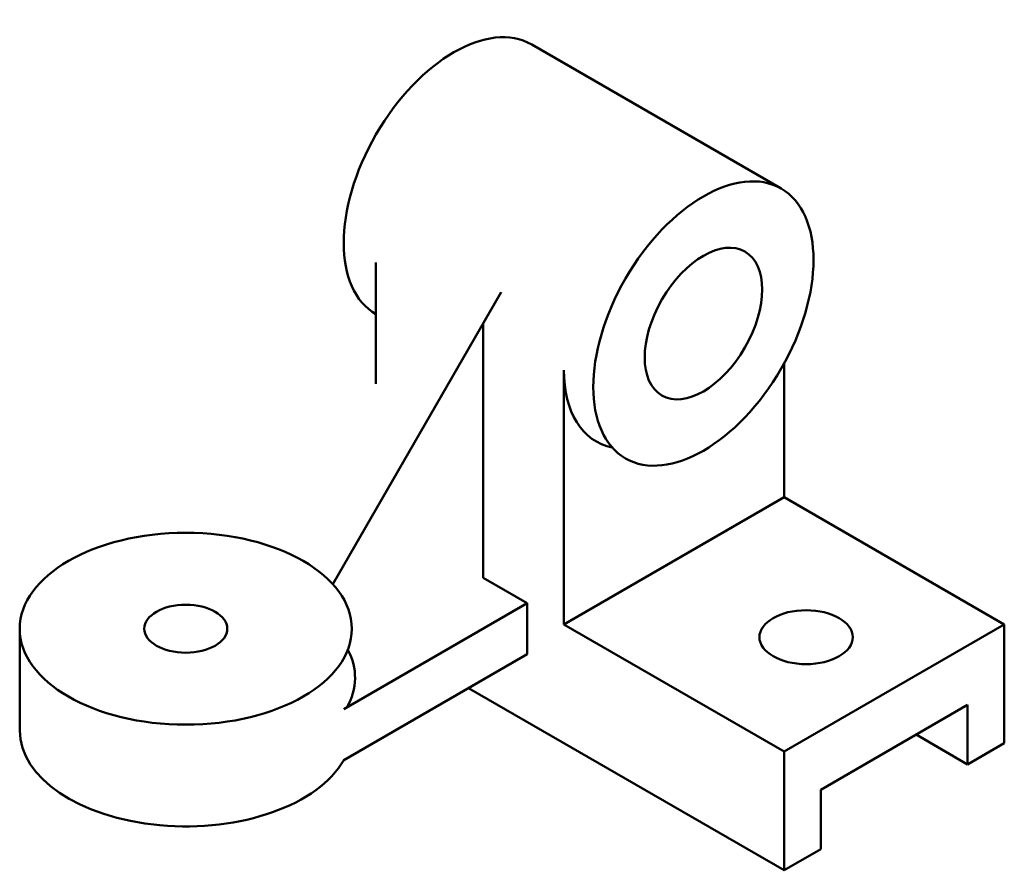
# Model space of a CAD drawing. Units: inches. Extents: x 77 to 4728, y 97 to 6127.
# Tile 1 of 2: x 77 to 309, y 97 to 298. Entities that reach past the tile are written whole.
import ezdxf

# ---------------------------------------------------------------- set-up
doc = ezdxf.new("R2010")
doc.units = ezdxf.units.IN
doc.header["$MEASUREMENT"] = 0
doc.layers.add('M-OUTL', color=7, linetype='Continuous', lineweight=50)

msp = doc.modelspace()

# ---------------------------------------------------------------- linework, layer by layer
at = {"layer": 'M-OUTL'}
for p, q in [((197.59, 292.03), (256.48, 258.03)), ((160.85, 228.39), (160.85, 240.6)), ((150.65, 164.73), (190.42, 233.61)), ((160.85, 228.39), (160.85, 212)), ((186.14, 166.21), (186.14, 226.21)), ((257.16, 185.21), (257.16, 216.81)), ((205.2, 155.21), (205.2, 215.21)), ((205.2, 155.21), (257.16, 185.21)), ((257.16, 185.21), (309.12, 155.21)), ((186.14, 166.21), (196.54, 160.21)), ((196.54, 160.21), (153.24, 135.21)), ((196.54, 160.21), (196.54, 148.21)), ((76.77, 154.2), (76.77, 130.2)), ((257.16, 125.21), (205.2, 155.21)), ((257.16, 125.21), (309.12, 155.21)), ((309.12, 155.21), (309.12, 127.21)), ((196.54, 148.21), (153.24, 123.21)), ((257.16, 97.21), (182.68, 140.21)), ((300.46, 136.21), (265.82, 116.21)), ((300.46, 122.21), (300.46, 136.21)), ((300.46, 122.21), (288.34, 129.21)), ((309.12, 127.21), (300.46, 122.21)), ((257.16, 97.21), (257.16, 125.21)), ((265.82, 116.21), (265.82, 102.21)), ((257.16, 97.21), (265.82, 102.21))]:
    msp.add_line(p, q, dxfattribs=at)
for centre, major_axis, start_param, end_param in [((179.22, 260.21), (-18.37, -31.82), 3.141593, 6.283185), ((231.18, 230.21), (-18.37, -31.82), 5.497787, 6.472883), ((116.72, 142.64), (-39.19, 0), 9.110787, 9.721308), ((115.96, 130.2), (-39.19, 0), 6.283185, 9.110787)]:
    msp.add_ellipse(centre, major_axis=major_axis, ratio=0.57735, start_param=start_param, end_param=end_param, dxfattribs=at)
for centre, major_axis in [((238.11, 226.21), (-18.37, -31.82)), ((238.11, 226.21), (-9.8, -16.97)), ((115.96, 154.2), (-39.19, 0)), ((115.96, 154.2), (-9.8, 0)), ((262.35, 152.21), (-11.02, 0))]:
    msp.add_ellipse(centre, major_axis=major_axis, ratio=0.57735, dxfattribs=at)

doc.saveas('drawing.dxf')
